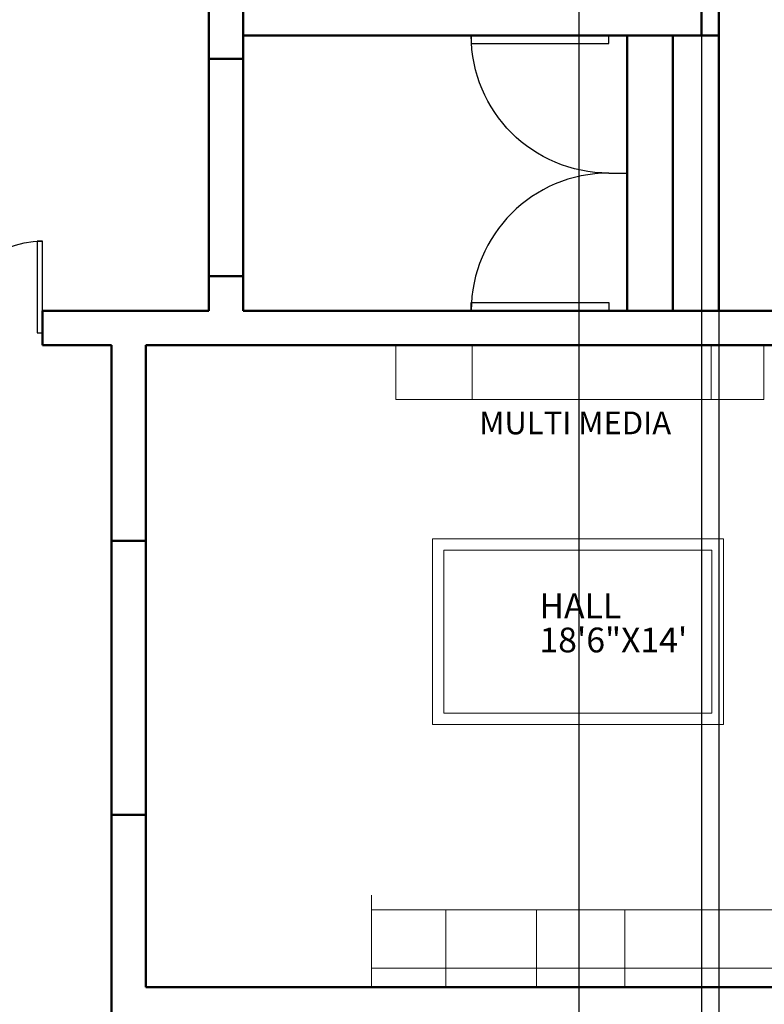
# Model space of a CAD drawing. Units: inches. Extents: x 5375 to 6084, y 16106 to 17259.
# Tile 25 of 32: x 5768 to 5963, y 16518 to 16776. Entities that reach past the tile are written whole.
import ezdxf

# ---------------------------------------------------------------- set-up
doc = ezdxf.new("R2010")
doc.units = ezdxf.units.IN
for name, color, linetype, lineweight in [('A-ANNO-DIMS', 2, 'Continuous', 18), ('A-ANNO-TEXT', 5, 'Continuous', 18), ('A-AREA-IDEN', 5, 'Continuous', 18), ('DOOR', 4, 'Continuous', 25), ('FURNITURE', 3, 'Continuous', 18), ('WALL', 6, 'Continuous', 50)]:
    doc.layers.add(name, color=color, linetype=linetype, lineweight=lineweight)
doc.styles.get("Standard").update_dxf_attribs({"font": 'arial.ttf'})
doc.dimstyles.get("Standard").update_dxf_attribs({"dimtxt": 0.18, "dimasz": 0.18, "dimexe": 0.18, "dimexo": 0.0625, "dimgap": 0.09, "dimtad": 0, "dimtih": 1, "dimtoh": 1, "dimdec": 4, "dimzin": 0, "dimdsep": 46, "dimtxsty": 'Standard', "dimcen": 0.09, "dimadec": 0, "dimazin": 0, "dimtfac": 1, "dimtdec": 4, "dimtofl": 0, "dimtmove": 0, "dimatfit": 3, "dimfxl": 1, "dimtolj": 1, "dimtzin": 0, "dimarcsym": 0})

# ---------------------------------------------------------------- blocks, each defined once
blk = doc.blocks.new('*U2')
for p, q in [((0, 0), (0, -100)), ((750, 0), (750, -100))]:
    blk.add_line(p, q)
blk.add_lwpolyline([(0, 0), (0, 750), (43.75, 750), (43.75, 0)], close=True)
blk.add_arc((0, 0), 750, 0, 90)
blk = doc.blocks.new('*D44')
at = {"layer": 'A-ANNO-DIMS', "color": 0, "lineweight": -2, "transparency": 16777216}
for p, q in [((5914, 16886.53), (5914, 16106.48)), ((5946.12, 16886.53), (5946.12, 16106.48)), ((5914.18, 16106.66), (5929.6, 16106.66)), ((5945.94, 16106.66), (5930.53, 16106.66))]:
    blk.add_line(p, q, dxfattribs=at)
at = {"layer": 'A-ANNO-DIMS', "color": 0, "transparency": 16777216}
for points in [[(5914.18, 16106.69), (5914.18, 16106.63), (5914, 16106.66)], [(5945.94, 16106.69), (5945.94, 16106.63), (5946.12, 16106.66)]]:
    blk.add_solid(points, dxfattribs=at)
at = {"layer": 'Defpoints', "color": 0, "transparency": 16777216}
for p in [(5914, 16886.6), (5946.12, 16886.6), (5914, 16106.66)]:
    blk.add_point(p, dxfattribs=at)
at = {"layer": 'A-ANNO-DIMS', "color": 0, "transparency": 16777216, "insert": (5930.06, 16106.66), "char_height": 0.18, "attachment_point": 5}
blk.add_mtext('\\A1;32.117', dxfattribs=at)
blk = doc.blocks.new('*D46')
at = {"layer": 'A-ANNO-DIMS', "color": 0, "lineweight": -2, "transparency": 16777216}
for p, q in [((5946.12, 16771.52), (5946.12, 16106.48)), ((5950.62, 16771.52), (5950.62, 16106.48)), ((5946.3, 16106.66), (5948.11, 16106.66)), ((5950.44, 16106.66), (5948.63, 16106.66))]:
    blk.add_line(p, q, dxfattribs=at)
at = {"layer": 'A-ANNO-DIMS', "color": 0, "transparency": 16777216}
for points in [[(5946.3, 16106.69), (5946.3, 16106.63), (5946.12, 16106.66)], [(5950.44, 16106.69), (5950.44, 16106.63), (5950.62, 16106.66)]]:
    blk.add_solid(points, dxfattribs=at)
at = {"layer": 'Defpoints', "color": 0, "transparency": 16777216}
for p in [(5946.12, 16771.58), (5950.62, 16771.58), (5950.62, 16106.66)]:
    blk.add_point(p, dxfattribs=at)
at = {"layer": 'A-ANNO-DIMS', "color": 0, "transparency": 16777216, "insert": (5948.37, 16106.66), "char_height": 0.18, "attachment_point": 5}
blk.add_mtext('\\A1;4.5', dxfattribs=at)

msp = doc.modelspace()

# ---------------------------------------------------------------- linework, layer by layer
at = {"layer": 'FURNITURE'}
for p, q in [((5886.0696, 16676.3446), (5886.0696, 16690.5793)), ((5948.5805, 16676.3446), (5948.5805, 16690.5793)), ((5859.7483, 16546.6662), (5859.7483, 16522.5793)), ((5859.7483, 16542.8395), (5994.1715, 16542.8395)), ((5879.1587, 16522.5793), (5879.1587, 16542.8395)), ((5902.8824, 16522.5793), (5902.8824, 16542.8395)), ((5926.0414, 16522.5793), (5926.0414, 16542.8395)), ((5950.6334, 16522.5793), (5950.6334, 16542.8395)), ((5859.7483, 16527.5002), (5974.4168, 16527.5002)), ((5859.7483, 16522.5793), (6001.018, 16522.5793))]:
    msp.add_line(p, q, dxfattribs=at)
for points in [[(5866.0498, 16690.5793), (5962.4336, 16690.5793), (5962.4336, 16676.3446), (5866.0498, 16676.3446)], [(5875.6754, 16639.9034), (5951.8163, 16639.9034), (5951.8163, 16591.259), (5875.6754, 16591.259)], [(5878.6754, 16636.9034), (5948.8163, 16636.9034), (5948.8163, 16594.259), (5878.6754, 16594.259)]]:
    msp.add_lwpolyline(points, close=True, dxfattribs=at)
at = {"layer": 'WALL'}
for p, q in [((5946.1199, 16891.5793), (5946.1199, 16771.5793)), ((5817.1199, 16879.5793), (5817.1199, 16699.5793)), ((5826.1199, 16879.5793), (5826.1199, 16699.5793)), ((5950.6199, 16828.5793), (5950.6199, 16699.5793)), ((5826.1199, 16771.5793), (5950.6199, 16771.5793)), ((5926.6199, 16771.5793), (5926.6199, 16699.5793)), ((5938.6199, 16771.5793), (5938.6199, 16699.5793)), ((5817.1199, 16765.491), (5826.1199, 16765.491)), ((5817.1199, 16708.6072), (5826.1199, 16708.6072)), ((5773.6199, 16690.5793), (5773.6199, 16699.5793)), ((5773.6199, 16699.5793), (5817.1199, 16699.5793)), ((5826.1199, 16699.5793), (5950.6199, 16699.5793)), ((5950.6199, 16699.5793), (6031.6199, 16699.5793)), ((5773.6199, 16690.5793), (5791.6199, 16690.5793)), ((5791.6199, 16690.5793), (5791.6199, 16513.5793)), ((5800.6199, 16690.5793), (5800.6199, 16522.5793)), ((5800.6199, 16690.5793), (6022.6199, 16690.5793)), ((5791.6199, 16639.3278), (5800.6199, 16639.3278)), ((5791.6199, 16567.6812), (5800.6199, 16567.6812)), ((5800.6199, 16522.5793), (6022.6199, 16522.5793))]:
    msp.add_line(p, q, dxfattribs=at)

# ---------------------------------------------------------------- block references
at = {"layer": 'DOOR', "yscale": 0.0479999999999998, "zscale": 0.0479999999999998, "rotation": 90}
for p, xscale in [((5921.8199, 16771.5793), -0.0479999999999998), ((5921.8199, 16699.5793), 0.0479999999999998)]:
    msp.add_blockref('*U2', p, dxfattribs=dict(at, xscale=xscale))
at = {"layer": 'DOOR', "xscale": -0.0319999999999999, "yscale": 0.0319999999999999, "zscale": 0.0319999999999999}
msp.add_blockref('*U2', (5773.6199, 16693.7793), dxfattribs=at)

# ---------------------------------------------------------------- texts
at = {"layer": 'A-ANNO-TEXT'}
msp.add_text('MULTI MEDIA', height=5.955513, dxfattribs=at).set_placement((5887.9097, 16667.2367))
at = {"layer": 'A-AREA-IDEN'}
for s, p in [('HALL', (5903.6631, 16619.1008)), ('18\'6"X14\'', (5903.6631, 16610.1677))]:
    msp.add_text(s, height=6.47981, dxfattribs=at).set_placement(p)

# ---------------------------------------------------------------- dimensions: what is measured, and where the dimension line sits
at = {"layer": 'A-ANNO-DIMS'}
for base, p1, p2, override, picture, middle in [((5914.0033, 16106.6631), (5946.1199, 16886.5956), (5914.0033, 16886.5956), {"dimdec": 3, "dimlfac": 1, "dimrnd": 0, "dimzin": 0, "dimdsep": 46, "dimlunit": 2}, '*D44', (5930.0616, 16106.6631)), ((5950.6199, 16106.6631), (5946.1199, 16771.5793), (5950.6199, 16771.5793), {"dimdec": 1, "dimlfac": 1, "dimrnd": 0, "dimzin": 0, "dimdsep": 46, "dimlunit": 2}, '*D46', (5948.3699, 16106.6631))]:
    dim = msp.add_linear_dim(base=base, p1=p1, p2=p2, dimstyle='Standard', override=override, dxfattribs=at)
    dim.commit()
    dim.dimension.update_dxf_attribs({"geometry": picture, "text_midpoint": middle})

doc.saveas('drawing.dxf')
